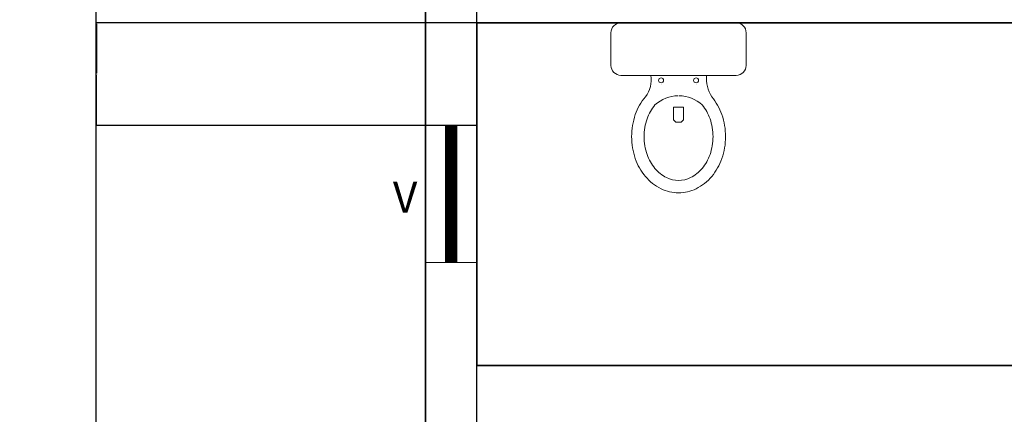
# Model space of a CAD drawing. Units: inches. Extents: x 318 to 927, y -1130 to 13.
# Tile 14 of 17: x 318 to 490, y -160 to -91. Entities that reach past the tile are written whole.
import ezdxf

# ---------------------------------------------------------------- set-up
doc = ezdxf.new("R2010")
doc.units = ezdxf.units.IN
doc.header["$MEASUREMENT"] = 0
for name, color, linetype, lineweight in [('A-ANNO-DIMS', 1, 'Continuous', 18), ('A-ANNO-IDEN', 1, 'Continuous', 13), ('A-FLOR-FIXT', 7, 'Continuous', 18), ('A-GLAZ-PATT', 5, 'Continuous', 9), ('wall', 1, 'Continuous', 35), ('win', 5, 'Continuous', 18)]:
    doc.layers.add(name, color=color, linetype=linetype, lineweight=lineweight)
doc.styles.get("Standard").update_dxf_attribs({"font": 'arial.ttf'})
doc.dimstyles.get("Standard").update_dxf_attribs({"dimtxt": 0.18, "dimasz": 0.18, "dimexe": 0.18, "dimexo": 0.0625, "dimgap": 0.09, "dimtad": 0, "dimtih": 1, "dimtoh": 1, "dimdec": 1, "dimzin": 0, "dimdsep": 46, "dimlunit": 4, "dimtxsty": 'Standard', "dimcen": 0.09, "dimadec": 0, "dimazin": 0, "dimtfac": 1, "dimtdec": 1, "dimtofl": 0, "dimtmove": 0, "dimatfit": 3, "dimfxl": 1, "dimtolj": 1, "dimtzin": 0, "dimarcsym": 0})

# ---------------------------------------------------------------- blocks, each defined once
blk = doc.blocks.new('WC-P01')
for p, q in [((-230, 0), (230, 0)), ((-270, -40), (-270, -170)), ((270, -40), (270, -170)), ((-230, -210), (230, -210)), ((-111.4, -210), (-111.4, -210)), ((-20, -337.8), (20, -337.8)), ((-20, -337.8), (-20, -385.7)), ((20, -337.8), (20, -385.7)), ((-18.5, -389.3), (-10.5, -397.3)), ((10.5, -397.3), (18.5, -389.3)), ((-10.5, -397.3), (10.5, -397.3))]:
    blk.add_line(p, q)
for points in [[(-111.4, -210, -0.215497), (-132.6, -295.9, 0.09084), (-172.8, -367.1, 0.083285), (-187.5, -455, 0.083285), (-172.8, -542.9, 0.09084), (-132.6, -614.1, 0.104065), (-70, -663.6, 0.115836), (0, -680, 0.115836), (70, -663.6, 0.104065), (132.6, -614.1, 0.09084), (172.8, -542.9, 0.083285), (187.5, -455, 0.083285)], [(187.5, -455, 0.083285), (172.8, -367.1, 0.09084), (132.6, -295.9, -0.156524), (111.4, -210)], [(-70, -246.4), (-70, -246.4, 0.104065)], [(70, -246.4), (70, -246.4, 0.115836)], [(-1.8, -291.3, 0.171753), (-94.2, -327.9, 0.09084), (-125.5, -383.5, 0.083285), (-137.5, -455, 0.083285), (-125.5, -526.5, 0.09084), (-94.2, -582.1, 0.104065), (-47.7, -618.8, 0.115836), (0, -630, 0.115836)], [(1.8, -291.3, -0.171753), (94.2, -327.9, -0.09084), (125.5, -383.5, -0.083285), (137.5, -455, -0.083285), (125.5, -526.5, -0.09084), (94.2, -582.1, -0.104065), (47.7, -618.8, -0.115836), (0, -630, -0.115836)]]:
    blk.add_lwpolyline(points, format="xyb")
for centre in [(-70, -230), (70, -230)]:
    blk.add_circle(centre, 10)
for centre, radius, start, end in [((-230, -40), 40, 90, 180), ((230, -40), 40, 0, 90), ((-230, -170), 40, 180, 270), ((230, -170), 40, 270, 0), ((-15, -385.7), 5, 180, 225), ((15, -385.7), 5, 315, 0)]:
    blk.add_arc(centre, radius, start, end)
blk = doc.blocks.new('_ArchTick')
at = {"color": 0, "linetype": 'ByBlock', "const_width": 0.15}
blk.add_lwpolyline([(-0.5, -0.5), (0.5, 0.5)], dxfattribs=at)
blk = doc.blocks.new('*D4')
at = {"layer": 'A-ANNO-DIMS', "color": 0, "lineweight": -2, "transparency": 16777216}
blk.add_line((331.26, -82.91), (331.26, -1042.91), dxfattribs=at)
at = {"layer": 'Defpoints', "color": 0, "transparency": 16777216}
for p in [(388.89, -82.91), (331.26, -1042.91), (388.89, -1042.91)]:
    blk.add_point(p, dxfattribs=at)
at = {"layer": 'A-ANNO-DIMS', "color": 0, "lineweight": -2, "transparency": 16777216, "xscale": 6, "yscale": 6, "zscale": 6}
for p, rotation in [((331.26, -82.91), 90), ((331.26, -1042.91), 270)]:
    blk.add_blockref('_ArchTick', p, dxfattribs=dict(at, rotation=rotation))
at = {"layer": 'A-ANNO-DIMS', "color": 0, "transparency": 16777216, "insert": (323.18, -562.91), "char_height": 8, "attachment_point": 5, "rotation": 90}
blk.add_mtext("\\A1;80'", dxfattribs=at)
blk = doc.blocks.new('VENT-24IN')
for p, q in [((9, 24), (0, 24)), ((3.5, 0), (3.5, 24)), ((5.5, 0), (5.5, 24)), ((9, 0), (0, 0))]:
    blk.add_line(p, q)
blk = doc.blocks.new('*D33')
at = {"layer": 'A-ANNO-DIMS', "color": 0, "lineweight": -2, "transparency": 16777216}
for p, q in [((397.89, -370.85), (397.89, -25.23)), ((398.07, -25.41), (464.5, -25.41)), ((531.71, -25.41), (465.28, -25.41)), ((531.89, -370.85), (531.89, -25.23))]:
    blk.add_line(p, q, dxfattribs=at)
at = {"layer": 'A-ANNO-DIMS', "color": 0, "transparency": 16777216}
for points in [[(398.07, -25.38), (398.07, -25.44), (397.89, -25.41)], [(531.71, -25.38), (531.71, -25.44), (531.89, -25.41)]]:
    blk.add_solid(points, dxfattribs=at)
at = {"layer": 'Defpoints', "color": 0, "transparency": 16777216}
for p in [(531.89, -25.41), (397.89, -370.91), (531.89, -370.91)]:
    blk.add_point(p, dxfattribs=at)
at = {"layer": 'A-ANNO-DIMS', "color": 0, "transparency": 16777216, "insert": (464.89, -25.41), "char_height": 0.18, "attachment_point": 5}
blk.add_mtext('\\A1;11\'-2"', dxfattribs=at)
blk = doc.blocks.new('*D65')
at = {"layer": 'A-ANNO-DIMS', "color": 0, "lineweight": -2, "transparency": 16777216}
for p, q in [((397.83, -91.91), (331.21, -91.91)), ((331.39, -92.09), (331.39, -100.73)), ((331.39, -109.73), (331.39, -101.09)), ((397.83, -109.91), (331.21, -109.91))]:
    blk.add_line(p, q, dxfattribs=at)
at = {"layer": 'A-ANNO-DIMS', "color": 0, "transparency": 16777216}
for points in [[(331.36, -92.09), (331.42, -92.09), (331.39, -91.91)], [(331.36, -109.73), (331.42, -109.73), (331.39, -109.91)]]:
    blk.add_solid(points, dxfattribs=at)
at = {"layer": 'Defpoints', "color": 0, "transparency": 16777216}
for p in [(397.89, -91.91), (331.39, -109.91), (397.89, -109.91)]:
    blk.add_point(p, dxfattribs=at)
at = {"layer": 'A-ANNO-DIMS', "color": 0, "transparency": 16777216, "insert": (331.39, -100.91), "char_height": 0.18, "attachment_point": 5}
blk.add_mtext('\\A1;1\'-6"', dxfattribs=at)

msp = doc.modelspace()

# ---------------------------------------------------------------- hatches: boundary and pattern name
at = {"layer": 'A-GLAZ-PATT'}
h = msp.add_hatch(dxfattribs=at)
h.set_pattern_fill('ANSI31', color=256)
h.paths.add_polyline_path([(394.39, -636.41), (392.39, -636.41), (392.39, -684.41), (394.39, -684.41)])
h.paths.add_polyline_path([(394.39, -319.91), (392.39, -319.91), (392.39, -343.91), (394.39, -343.91)])
h.paths.add_polyline_path([(394.39, -172.63), (392.39, -172.63), (392.39, -208.63), (394.39, -208.63)])
h.paths.add_polyline_path([(394.39, -109.91), (392.39, -109.91), (392.39, -133.91), (394.39, -133.91)])
h.paths.add_polyline_path([(865.39, -102.49), (863.39, -102.49), (863.39, -138.49), (865.39, -138.49)])

# ---------------------------------------------------------------- linework, layer by layer
at = {"layer": 'wall'}
for p, q in [((388.89, -82.91), (388.89, -1042.91)), ((397.89, -91.91), (397.89, -151.91)), ((589.89, -91.91), (397.89, -91.91)), ((551.89, -151.91), (397.89, -151.91))]:
    msp.add_line(p, q, dxfattribs=at)

# ---------------------------------------------------------------- block references
at = {"layer": 'A-FLOR-FIXT', "xscale": 0.0438047028060103, "yscale": 0.0438047028060103, "zscale": 0.0438047028060103}
msp.add_blockref('WC-P01', (433.17, -91.91), dxfattribs=at)
at = {"layer": 'win'}
msp.add_blockref('VENT-24IN', (388.89, -133.91), dxfattribs=at)

# ---------------------------------------------------------------- texts
at = {"layer": 'A-ANNO-IDEN'}
msp.add_text('V', height=5.44, dxfattribs=at).set_placement((383.21, -125.16))

# ---------------------------------------------------------------- dimensions: what is measured, and where the dimension line sits
at = {"layer": 'A-ANNO-DIMS'}
dim = msp.add_linear_dim(base=(531.89, -25.41), p1=(397.89, -370.91), p2=(531.89, -370.91), dimstyle='Standard', override={"dimdec": 1, "dimlfac": 1, "dimrnd": 0, "dimzin": 1, "dimdsep": 46, "dimlunit": 4, "dimfrac": 2}, dxfattribs=at)
dim.commit()
dim.dimension.update_dxf_attribs({"geometry": '*D33', "text_midpoint": (464.89, -25.41)})
for base, p1, p2, override, picture, middle in [((331.26, -1042.91), (388.89, -82.91), (388.89, -1042.91), {"dimtxt": 8, "dimasz": 6, "dimgap": 4, "dimtad": 1, "dimtih": 0, "dimblk1": 'ArchTick', "dimblk2": 'ArchTick', "dimsah": 1, "dimse1": 1, "dimse2": 1, "dimclrd": 0, "dimclre": 0, "dimclrt": 0}, '*D4', (323.18, -562.91)), ((331.39, -109.91), (397.89, -91.91), (397.89, -109.91), {"dimdec": 1, "dimlfac": 1, "dimrnd": 0, "dimzin": 1, "dimdsep": 46, "dimlunit": 4, "dimfrac": 2}, '*D65', (331.39, -100.91))]:
    dim = msp.add_linear_dim(base=base, p1=p1, p2=p2, angle=90, dimstyle='Standard', override=override, dxfattribs=at)
    dim.commit()
    dim.dimension.update_dxf_attribs({"geometry": picture, "text_midpoint": middle})

doc.saveas('drawing.dxf')
